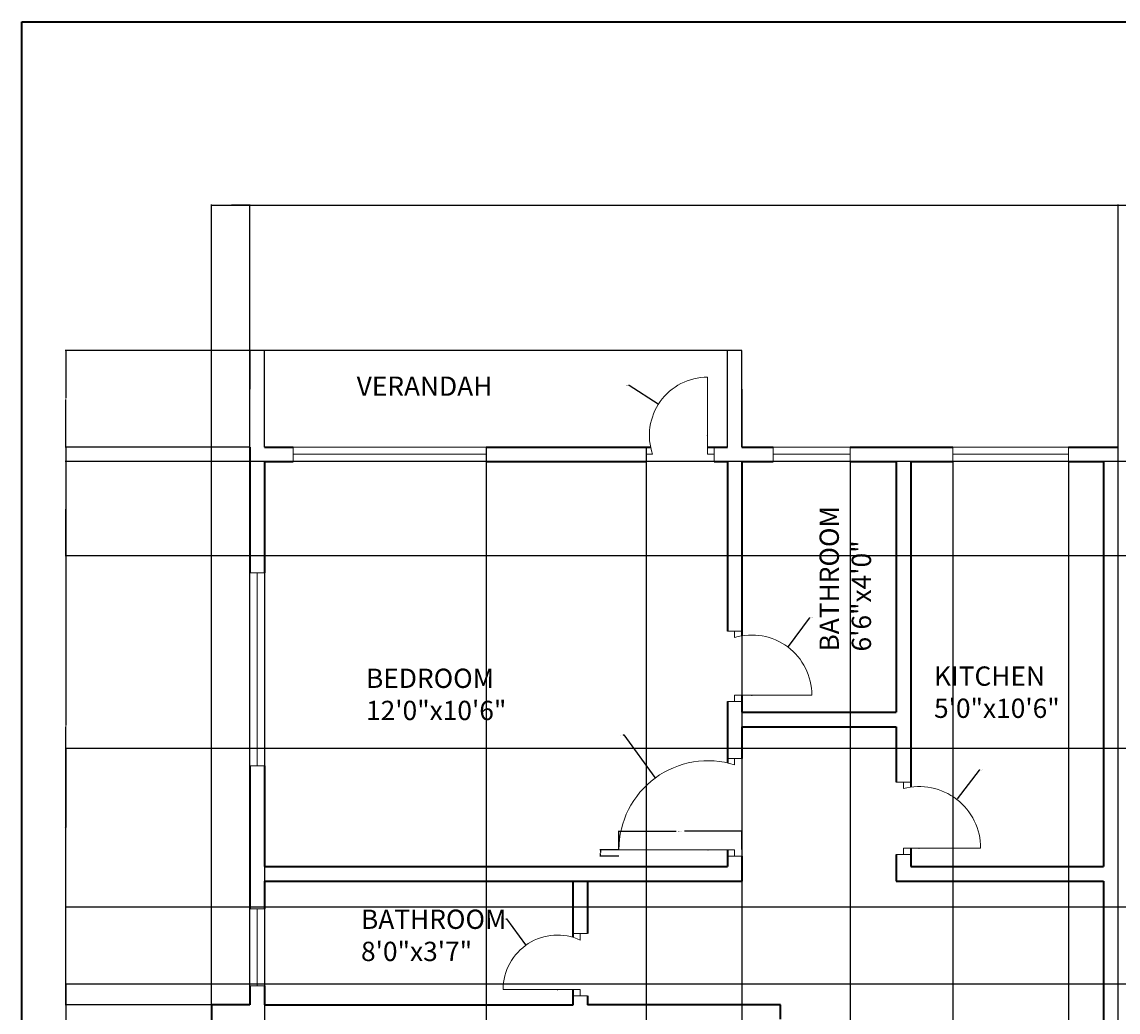
# Model space of a CAD drawing. Units: inches. Extents: x 1831 to 2867, y 1605 to 2524.
# Tile 4 of 7: x 1831 to 2172, y 2216 to 2524. Entities that reach past the tile are written whole.
import ezdxf

# ---------------------------------------------------------------- set-up
doc = ezdxf.new("R2010")
doc.units = ezdxf.units.IN
for name, color, linetype, lineweight in [('A-ANNO-DIMS', 2, 'Continuous', 18), ('A-ANNO-TTLB', 7, 'Continuous', 35), ('A-AREA-IDEN', 7, 'Continuous', 18), ('A-DOOR', 11, 'Continuous', 18), ('A-FLOR-BALC', 7, 'Continuous', 25), ('A-GLAZ', 121, 'Continuous', 18), ('A-WALL', 7, 'Continuous', 35)]:
    doc.layers.add(name, color=color, linetype=linetype, lineweight=lineweight)
doc.styles.get("Standard").update_dxf_attribs({"font": 'arial.ttf'})
doc.dimstyles.get("Standard").update_dxf_attribs({"dimtxt": 0.18, "dimasz": 0.18, "dimexe": 0.18, "dimexo": 0.0625, "dimgap": 0.09, "dimtad": 0, "dimtih": 1, "dimtoh": 1, "dimdec": 4, "dimzin": 0, "dimdsep": 46, "dimtxsty": 'Standard', "dimcen": 0.09, "dimadec": 0, "dimazin": 0, "dimtfac": 1, "dimtdec": 4, "dimtofl": 0, "dimtmove": 0, "dimatfit": 3, "dimfxl": 1, "dimtolj": 1, "dimtzin": 0, "dimarcsym": 0})

# ---------------------------------------------------------------- blocks, each defined once
blk = doc.blocks.new('WIN-60IN')
for p, q in [((4.5, 60), (0, 60)), ((0, 60), (2.25, 60)), ((0, 0), (0, 60)), ((2.25, 60), (2.25, 0)), ((4.5, 60), (4.5, 0)), ((4.5, 0), (0, 0)), ((2.25, 0), (4.5, 0))]:
    blk.add_line(p, q)
blk = doc.blocks.new('DOOR-LEAF-36IN-ALT')
for p, q in [((36, 2), (0, 2)), ((33.75, 0), (38.25, 0)), ((36, 0), (36, 2)), ((38.25, 0), (36, 0))]:
    blk.add_line(p, q)
blk = doc.blocks.new('DOOR-LEAF-24IN')
for p, q in [((2.25, 0), (2.25, 2)), ((2.25, 2), (26.25, 2)), ((0, 0), (4.5, 0)), ((4.5, 0), (2.25, 0))]:
    blk.add_line(p, q)
blk = doc.blocks.new('DOOR-LEAF-24IN-ALT')
for p, q in [((24, 2), (0, 2)), ((21.75, 0), (26.25, 0)), ((24, 0), (24, 2)), ((26.25, 0), (24, 0))]:
    blk.add_line(p, q)
blk = doc.blocks.new('DOOR-STRIKE-JAMB')
for p, q in [((0, 0), (4.5, 0)), ((2.25, 0), (2.25, 2)), ((4.5, 0), (2.25, 0))]:
    blk.add_line(p, q)
blk = doc.blocks.new('*D12')
at = {"layer": 'A-ANNO-DIMS', "color": 0, "lineweight": -2, "transparency": 16777216}
for p, q in [((2016.8, 2266.47), (2016.8, 2272.33)), ((2016.98, 2272.15), (2034.64, 2272.15)), ((2054.87, 2272.15), (2037.21, 2272.15)), ((2055.05, 2266.47), (2055.05, 2272.33))]:
    blk.add_line(p, q, dxfattribs=at)
at = {"layer": 'A-ANNO-DIMS', "color": 0, "transparency": 16777216}
for points in [[(2016.98, 2272.18), (2016.98, 2272.12), (2016.8, 2272.15)], [(2054.87, 2272.18), (2054.87, 2272.12), (2055.05, 2272.15)]]:
    blk.add_solid(points, dxfattribs=at)
at = {"layer": 'Defpoints', "color": 0, "transparency": 16777216}
for p in [(2055.05, 2272.15), (2016.8, 2266.41), (2055.05, 2266.41)]:
    blk.add_point(p, dxfattribs=at)
at = {"layer": 'A-ANNO-DIMS', "color": 0, "transparency": 16777216, "insert": (2035.93, 2272.15), "char_height": 0.18, "attachment_point": 5}
blk.add_mtext('\\A1;DOOR LEAF 38 TYP.', dxfattribs=at)
blk = doc.blocks.new('*D13')
at = {"layer": 'A-ANNO-DIMS', "color": 0, "lineweight": -2, "transparency": 16777216}
for p, q in [((2016.74, 2266.41), (2010.88, 2266.41)), ((2016.74, 2264.41), (2010.88, 2264.41)), ((2011.06, 2266.23), (2011.06, 2265.59)), ((2011.06, 2264.59), (2011.06, 2265.23))]:
    blk.add_line(p, q, dxfattribs=at)
at = {"layer": 'A-ANNO-DIMS', "color": 0, "transparency": 16777216}
for points in [[(2011.03, 2266.23), (2011.09, 2266.23), (2011.06, 2266.41)], [(2011.03, 2264.59), (2011.09, 2264.59), (2011.06, 2264.41)]]:
    blk.add_solid(points, dxfattribs=at)
at = {"layer": 'Defpoints', "color": 0, "transparency": 16777216}
for p in [(2011.06, 2266.41), (2016.8, 2266.41), (2016.8, 2264.41)]:
    blk.add_point(p, dxfattribs=at)
at = {"layer": 'A-ANNO-DIMS', "color": 0, "transparency": 16777216, "insert": (2011.06, 2265.41), "char_height": 0.18, "attachment_point": 5}
blk.add_mtext('\\A1;2 TYP.', dxfattribs=at)
blk = doc.blocks.new('*D22')
at = {"layer": 'A-ANNO-DIMS', "color": 0, "lineweight": -2, "transparency": 16777216}
for p, q in [((1890.05, 2218.24), (1890.05, 2467.15)), ((1890.23, 2466.97), (2341.22, 2466.97)), ((2792.79, 2466.97), (2341.8, 2466.97)), ((2792.97, 2421.74), (2792.97, 2467.15))]:
    blk.add_line(p, q, dxfattribs=at)
at = {"layer": 'A-ANNO-DIMS', "color": 0, "transparency": 16777216}
for points in [[(1890.23, 2467), (1890.23, 2466.94), (1890.05, 2466.97)], [(2792.79, 2467), (2792.79, 2466.94), (2792.97, 2466.97)]]:
    blk.add_solid(points, dxfattribs=at)
at = {"layer": 'Defpoints', "color": 0, "transparency": 16777216}
for p in [(2792.97, 2466.97), (2792.97, 2421.67), (1890.05, 2218.17)]:
    blk.add_point(p, dxfattribs=at)
at = {"layer": 'A-ANNO-DIMS', "color": 0, "transparency": 16777216, "insert": (2341.51, 2466.97), "char_height": 0.18, "attachment_point": 5}
blk.add_mtext('\\A1;903', dxfattribs=at)
blk = doc.blocks.new('*D31')
at = {"layer": 'A-ANNO-DIMS', "color": 0, "lineweight": -2, "transparency": 16777216}
for p, q in [((1901.99, 2421.67), (1844.57, 2421.67)), ((1844.75, 2421.49), (1844.75, 2406.86)), ((1844.75, 2391.85), (1844.75, 2406.49)), ((1901.99, 2391.67), (1844.57, 2391.67))]:
    blk.add_line(p, q, dxfattribs=at)
at = {"layer": 'A-ANNO-DIMS', "color": 0, "transparency": 16777216}
for points in [[(1844.72, 2421.49), (1844.78, 2421.49), (1844.75, 2421.67)], [(1844.72, 2391.85), (1844.78, 2391.85), (1844.75, 2391.67)]]:
    blk.add_solid(points, dxfattribs=at)
at = {"layer": 'Defpoints', "color": 0, "transparency": 16777216}
for p in [(1902.05, 2421.67), (1844.75, 2391.67), (1902.05, 2391.67)]:
    blk.add_point(p, dxfattribs=at)
at = {"layer": 'A-ANNO-DIMS', "color": 0, "transparency": 16777216, "insert": (1844.75, 2406.67), "char_height": 0.18, "attachment_point": 5}
blk.add_mtext('\\A1;30', dxfattribs=at)
blk = doc.blocks.new('*D32')
at = {"layer": 'A-ANNO-DIMS', "color": 0, "lineweight": -2, "transparency": 16777216}
for p, q in [((1901.99, 2391.67), (1844.57, 2391.67)), ((1844.75, 2391.49), (1844.75, 2305.11)), ((1844.75, 2218.35), (1844.75, 2304.74)), ((1901.99, 2218.17), (1844.57, 2218.17))]:
    blk.add_line(p, q, dxfattribs=at)
at = {"layer": 'A-ANNO-DIMS', "color": 0, "transparency": 16777216}
for points in [[(1844.72, 2391.49), (1844.78, 2391.49), (1844.75, 2391.67)], [(1844.72, 2218.35), (1844.78, 2218.35), (1844.75, 2218.17)]]:
    blk.add_solid(points, dxfattribs=at)
at = {"layer": 'Defpoints', "color": 0, "transparency": 16777216}
for p in [(1902.05, 2391.67), (1844.75, 2218.17), (1902.05, 2218.17)]:
    blk.add_point(p, dxfattribs=at)
at = {"layer": 'A-ANNO-DIMS', "color": 0, "transparency": 16777216, "insert": (1844.75, 2304.92), "char_height": 0.18, "attachment_point": 5}
blk.add_mtext('\\A1;173.5', dxfattribs=at)
blk = doc.blocks.new('*D33')
at = {"layer": 'A-ANNO-DIMS', "color": 0, "lineweight": -2, "transparency": 16777216}
for p, q in [((1889.99, 2218.17), (1844.57, 2218.17)), ((1844.75, 2217.99), (1844.75, 2093.86)), ((1844.75, 1969.35), (1844.75, 2093.49)), ((1889.99, 1969.17), (1844.57, 1969.17))]:
    blk.add_line(p, q, dxfattribs=at)
at = {"layer": 'A-ANNO-DIMS', "color": 0, "transparency": 16777216}
for points in [[(1844.72, 2217.99), (1844.78, 2217.99), (1844.75, 2218.17)], [(1844.72, 1969.35), (1844.78, 1969.35), (1844.75, 1969.17)]]:
    blk.add_solid(points, dxfattribs=at)
at = {"layer": 'Defpoints', "color": 0, "transparency": 16777216}
for p in [(1890.05, 2218.17), (1844.75, 1969.17), (1890.05, 1969.17)]:
    blk.add_point(p, dxfattribs=at)
at = {"layer": 'A-ANNO-DIMS', "color": 0, "transparency": 16777216, "insert": (1844.75, 2093.67), "char_height": 0.18, "attachment_point": 5}
blk.add_mtext('\\A1;249', dxfattribs=at)
blk = doc.blocks.new('*D36')
at = {"layer": 'A-ANNO-DIMS', "color": 0, "lineweight": -2, "transparency": 16777216}
for p, q in [((1890.05, 2218.24), (1890.05, 2467.15)), ((1890.23, 2466.97), (1895.84, 2466.97)), ((1901.87, 2466.97), (1896.26, 2466.97)), ((1902.05, 2218.24), (1902.05, 2467.15))]:
    blk.add_line(p, q, dxfattribs=at)
at = {"layer": 'A-ANNO-DIMS', "color": 0, "transparency": 16777216}
for points in [[(1890.23, 2467), (1890.23, 2466.94), (1890.05, 2466.97)], [(1901.87, 2467), (1901.87, 2466.94), (1902.05, 2466.97)]]:
    blk.add_solid(points, dxfattribs=at)
at = {"layer": 'Defpoints', "color": 0, "transparency": 16777216}
for p in [(1902.05, 2466.97), (1890.05, 2218.17), (1902.05, 2218.17)]:
    blk.add_point(p, dxfattribs=at)
at = {"layer": 'A-ANNO-DIMS', "color": 0, "transparency": 16777216, "insert": (1896.05, 2466.97), "char_height": 0.18, "attachment_point": 5}
blk.add_mtext('\\A1;12', dxfattribs=at)
blk = doc.blocks.new('*D37')
at = {"layer": 'A-ANNO-DIMS', "color": 0, "lineweight": -2, "transparency": 16777216}
for p, q in [((1906.55, 2387.11), (1906.55, 1715.69)), ((1975.47, 2387.11), (1975.47, 1715.69)), ((1906.73, 1715.87), (1940.62, 1715.87)), ((1975.29, 1715.87), (1941.4, 1715.87))]:
    blk.add_line(p, q, dxfattribs=at)
at = {"layer": 'A-ANNO-DIMS', "color": 0, "transparency": 16777216}
for points in [[(1906.73, 1715.9), (1906.73, 1715.84), (1906.55, 1715.87)], [(1975.29, 1715.9), (1975.29, 1715.84), (1975.47, 1715.87)]]:
    blk.add_solid(points, dxfattribs=at)
at = {"layer": 'Defpoints', "color": 0, "transparency": 16777216}
for p in [(1906.55, 2387.17), (1975.47, 2387.17), (1975.47, 1715.87)]:
    blk.add_point(p, dxfattribs=at)
at = {"layer": 'A-ANNO-DIMS', "color": 0, "transparency": 16777216, "insert": (1941.01, 1715.87), "char_height": 0.18, "attachment_point": 5}
blk.add_mtext('\\A1;68.92', dxfattribs=at)
blk = doc.blocks.new('*D38')
at = {"layer": 'A-ANNO-DIMS', "color": 0, "lineweight": -2, "transparency": 16777216}
for p, q in [((1975.47, 2391.61), (1975.47, 1715.69)), ((2025.28, 2391.61), (2025.28, 1715.69)), ((1975.65, 1715.87), (1999.99, 1715.87)), ((2025.1, 1715.87), (2000.75, 1715.87))]:
    blk.add_line(p, q, dxfattribs=at)
at = {"layer": 'A-ANNO-DIMS', "color": 0, "transparency": 16777216}
for points in [[(1975.65, 1715.9), (1975.65, 1715.84), (1975.47, 1715.87)], [(2025.1, 1715.9), (2025.1, 1715.84), (2025.28, 1715.87)]]:
    blk.add_solid(points, dxfattribs=at)
at = {"layer": 'Defpoints', "color": 0, "transparency": 16777216}
for p in [(1975.47, 2391.67), (2025.28, 2391.67), (2025.28, 1715.87)]:
    blk.add_point(p, dxfattribs=at)
at = {"layer": 'A-ANNO-DIMS', "color": 0, "transparency": 16777216, "insert": (2000.37, 1715.87), "char_height": 0.18, "attachment_point": 5}
blk.add_mtext('\\A1;49.81', dxfattribs=at)
blk = doc.blocks.new('*D39')
at = {"layer": 'A-ANNO-DIMS', "color": 0, "lineweight": -2, "transparency": 16777216}
for p, q in [((2055.05, 2387.11), (2055.05, 1715.69)), ((2088.73, 2387.11), (2088.73, 1715.69)), ((2055.23, 1715.87), (2071.5, 1715.87)), ((2088.55, 1715.87), (2072.28, 1715.87))]:
    blk.add_line(p, q, dxfattribs=at)
at = {"layer": 'A-ANNO-DIMS', "color": 0, "transparency": 16777216}
for points in [[(2055.23, 1715.9), (2055.23, 1715.84), (2055.05, 1715.87)], [(2088.55, 1715.9), (2088.55, 1715.84), (2088.73, 1715.87)]]:
    blk.add_solid(points, dxfattribs=at)
at = {"layer": 'Defpoints', "color": 0, "transparency": 16777216}
for p in [(2055.05, 2387.17), (2088.73, 2387.17), (2088.73, 1715.87)]:
    blk.add_point(p, dxfattribs=at)
at = {"layer": 'A-ANNO-DIMS', "color": 0, "transparency": 16777216, "insert": (2071.89, 1715.87), "char_height": 0.18, "attachment_point": 5}
blk.add_mtext('\\A1;33.68', dxfattribs=at)
blk = doc.blocks.new('*D40')
at = {"layer": 'A-ANNO-DIMS', "color": 0, "lineweight": -2, "transparency": 16777216}
for p, q in [((2088.73, 2387.11), (2088.73, 1715.69)), ((2120.64, 2387.11), (2120.64, 1715.69)), ((2088.91, 1715.87), (2104.31, 1715.87)), ((2120.46, 1715.87), (2105.06, 1715.87))]:
    blk.add_line(p, q, dxfattribs=at)
at = {"layer": 'A-ANNO-DIMS', "color": 0, "transparency": 16777216}
for points in [[(2088.91, 1715.9), (2088.91, 1715.84), (2088.73, 1715.87)], [(2120.46, 1715.9), (2120.46, 1715.84), (2120.64, 1715.87)]]:
    blk.add_solid(points, dxfattribs=at)
at = {"layer": 'Defpoints', "color": 0, "transparency": 16777216}
for p in [(2088.73, 2387.17), (2120.64, 2387.17), (2120.64, 1715.87)]:
    blk.add_point(p, dxfattribs=at)
at = {"layer": 'A-ANNO-DIMS', "color": 0, "transparency": 16777216, "insert": (2104.69, 1715.87), "char_height": 0.18, "attachment_point": 5}
blk.add_mtext('\\A1;31.91', dxfattribs=at)
blk = doc.blocks.new('*D41')
at = {"layer": 'A-ANNO-DIMS', "color": 0, "lineweight": -2, "transparency": 16777216}
for p, q in [((2156.64, 2387.11), (2156.64, 1715.69)), ((2210.17, 2387.11), (2210.17, 1715.69)), ((2156.82, 1715.87), (2183.01, 1715.87)), ((2209.99, 1715.87), (2183.8, 1715.87))]:
    blk.add_line(p, q, dxfattribs=at)
at = {"layer": 'A-ANNO-DIMS', "color": 0, "transparency": 16777216}
for points in [[(2156.82, 1715.9), (2156.82, 1715.84), (2156.64, 1715.87)], [(2209.99, 1715.9), (2209.99, 1715.84), (2210.17, 1715.87)]]:
    blk.add_solid(points, dxfattribs=at)
at = {"layer": 'Defpoints', "color": 0, "transparency": 16777216}
for p in [(2156.64, 2387.17), (2210.17, 2387.17), (2210.17, 1715.87)]:
    blk.add_point(p, dxfattribs=at)
at = {"layer": 'A-ANNO-DIMS', "color": 0, "transparency": 16777216, "insert": (2183.4, 1715.87), "char_height": 0.18, "attachment_point": 5}
blk.add_mtext('\\A1;53.52', dxfattribs=at)
blk = doc.blocks.new('*D49')
at = {"layer": 'A-ANNO-DIMS', "color": 0, "lineweight": -2, "transparency": 16777216}
for p, q in [((2786.99, 2387.17), (1844.57, 2387.17)), ((1844.75, 2386.99), (1844.75, 2372.7)), ((1844.75, 2358.05), (1844.75, 2372.34)), ((2786.99, 2357.87), (1844.57, 2357.87))]:
    blk.add_line(p, q, dxfattribs=at)
at = {"layer": 'A-ANNO-DIMS', "color": 0, "transparency": 16777216}
for points in [[(1844.72, 2386.99), (1844.78, 2386.99), (1844.75, 2387.17)], [(1844.72, 2358.05), (1844.78, 2358.05), (1844.75, 2357.87)]]:
    blk.add_solid(points, dxfattribs=at)
at = {"layer": 'Defpoints', "color": 0, "transparency": 16777216}
for p in [(2787.05, 2387.17), (1844.75, 2357.87), (2787.05, 2357.87)]:
    blk.add_point(p, dxfattribs=at)
at = {"layer": 'A-ANNO-DIMS', "color": 0, "transparency": 16777216, "insert": (1844.75, 2372.52), "char_height": 0.18, "attachment_point": 5}
blk.add_mtext('\\A1;29.31', dxfattribs=at)
blk = doc.blocks.new('*D50')
at = {"layer": 'A-ANNO-DIMS', "color": 0, "lineweight": -2, "transparency": 16777216}
for p, q in [((2786.99, 2297.87), (1844.57, 2297.87)), ((1844.75, 2297.69), (1844.75, 2273.42)), ((1844.75, 2248.78), (1844.75, 2273.05)), ((2786.99, 2248.6), (1844.57, 2248.6))]:
    blk.add_line(p, q, dxfattribs=at)
at = {"layer": 'A-ANNO-DIMS', "color": 0, "transparency": 16777216}
for points in [[(1844.72, 2297.69), (1844.78, 2297.69), (1844.75, 2297.87)], [(1844.72, 2248.78), (1844.78, 2248.78), (1844.75, 2248.6)]]:
    blk.add_solid(points, dxfattribs=at)
at = {"layer": 'Defpoints', "color": 0, "transparency": 16777216}
for p in [(2787.05, 2297.87), (1844.75, 2248.6), (2787.05, 2248.6)]:
    blk.add_point(p, dxfattribs=at)
at = {"layer": 'A-ANNO-DIMS', "color": 0, "transparency": 16777216, "insert": (1844.75, 2273.23), "char_height": 0.18, "attachment_point": 5}
blk.add_mtext('\\A1;49.26', dxfattribs=at)
blk = doc.blocks.new('*D51')
at = {"layer": 'A-ANNO-DIMS', "color": 0, "lineweight": -2, "transparency": 16777216}
for p, q in [((2786.99, 2224.6), (1844.57, 2224.6)), ((1844.75, 2224.42), (1844.75, 2206.21)), ((1844.75, 2187.63), (1844.75, 2205.85)), ((2786.99, 2187.45), (1844.57, 2187.45))]:
    blk.add_line(p, q, dxfattribs=at)
at = {"layer": 'A-ANNO-DIMS', "color": 0, "transparency": 16777216}
for points in [[(1844.72, 2224.42), (1844.78, 2224.42), (1844.75, 2224.6)], [(1844.72, 2187.63), (1844.78, 2187.63), (1844.75, 2187.45)]]:
    blk.add_solid(points, dxfattribs=at)
at = {"layer": 'Defpoints', "color": 0, "transparency": 16777216}
for p in [(2787.05, 2224.6), (1844.75, 2187.45), (2787.05, 2187.45)]:
    blk.add_point(p, dxfattribs=at)
at = {"layer": 'A-ANNO-DIMS', "color": 0, "transparency": 16777216, "insert": (1844.75, 2206.03), "char_height": 0.18, "attachment_point": 5}
blk.add_mtext('\\A1;37.15', dxfattribs=at)
blk = doc.blocks.new('*D63')
at = {"layer": 'A-ANNO-DIMS', "color": 0, "lineweight": -2, "transparency": 16777216}
for p, q in [((2172.05, 1795.74), (2172.05, 2467.15)), ((2172.23, 2466.97), (2183.83, 2466.97)), ((2195.87, 2466.97), (2184.27, 2466.97)), ((2196.05, 1795.74), (2196.05, 2467.15))]:
    blk.add_line(p, q, dxfattribs=at)
at = {"layer": 'A-ANNO-DIMS', "color": 0, "transparency": 16777216}
for points in [[(2172.23, 2467), (2172.23, 2466.94), (2172.05, 2466.97)], [(2195.87, 2467), (2195.87, 2466.94), (2196.05, 2466.97)]]:
    blk.add_solid(points, dxfattribs=at)
at = {"layer": 'Defpoints', "color": 0, "transparency": 16777216}
for p in [(2196.05, 2466.97), (2172.05, 1795.67), (2196.05, 1795.67)]:
    blk.add_point(p, dxfattribs=at)
at = {"layer": 'A-ANNO-DIMS', "color": 0, "transparency": 16777216, "insert": (2184.05, 2466.97), "char_height": 0.18, "attachment_point": 5}
blk.add_mtext('\\A1;24', dxfattribs=at)
blk = doc.blocks.new('*D75')
at = {"layer": 'A-ANNO-DIMS', "color": 0, "lineweight": -2, "transparency": 16777216}
for p, q in [((2018.1, 2302.13), (2018.28, 2302.13)), ((2018.28, 2302.13), (2028, 2288.88)), ((2044.41, 2266.41), (2044.59, 2266.41)), ((2044.5, 2266.32), (2044.5, 2266.5))]:
    blk.add_line(p, q, dxfattribs=at)
at = {"layer": 'A-ANNO-DIMS', "color": 0, "transparency": 16777216}
blk.add_solid([(2028.03, 2288.9), (2027.98, 2288.86), (2028.11, 2288.74)], dxfattribs=at)
at = {"layer": 'Defpoints', "color": 0, "transparency": 16777216}
for p in [(2028.11, 2288.74), (2044.5, 2266.41)]:
    blk.add_point(p, dxfattribs=at)
at = {"layer": 'A-ANNO-DIMS', "color": 0, "transparency": 16777216, "insert": (2017.55, 2302.13), "char_height": 0.18, "attachment_point": 5}
blk.add_mtext('\\A1;R27.694', dxfattribs=at)
blk = doc.blocks.new('*D88')
at = {"layer": 'A-ANNO-DIMS', "color": 0, "lineweight": -2, "transparency": 16777216}
for p, q in [((2128.89, 2291.19), (2121.96, 2282.24)), ((2129.07, 2291.19), (2128.89, 2291.19)), ((2110.04, 2266.93), (2110.22, 2266.93)), ((2110.13, 2266.84), (2110.13, 2267.02))]:
    blk.add_line(p, q, dxfattribs=at)
at = {"layer": 'A-ANNO-DIMS', "color": 0, "transparency": 16777216}
blk.add_solid([(2121.94, 2282.25), (2121.99, 2282.22), (2121.85, 2282.09)], dxfattribs=at)
at = {"layer": 'Defpoints', "color": 0, "transparency": 16777216}
for p in [(2121.85, 2282.09), (2110.13, 2266.93)]:
    blk.add_point(p, dxfattribs=at)
at = {"layer": 'A-ANNO-DIMS', "color": 0, "transparency": 16777216, "insert": (2129.62, 2291.19), "char_height": 0.18, "attachment_point": 5}
blk.add_mtext('\\A1;R19.168', dxfattribs=at)
blk = doc.blocks.new('*D93')
at = {"layer": 'A-ANNO-DIMS', "color": 0, "lineweight": -2, "transparency": 16777216}
for p, q in [((2075.99, 2338.48), (2069.4, 2329.65)), ((2076.17, 2338.48), (2075.99, 2338.48)), ((2058.04, 2314.53), (2058.22, 2314.53)), ((2058.13, 2314.44), (2058.13, 2314.62))]:
    blk.add_line(p, q, dxfattribs=at)
at = {"layer": 'A-ANNO-DIMS', "color": 0, "transparency": 16777216}
blk.add_solid([(2069.37, 2329.66), (2069.42, 2329.63), (2069.29, 2329.5)], dxfattribs=at)
at = {"layer": 'Defpoints', "color": 0, "transparency": 16777216}
for p in [(2069.29, 2329.5), (2058.13, 2314.53)]:
    blk.add_point(p, dxfattribs=at)
at = {"layer": 'A-ANNO-DIMS', "color": 0, "transparency": 16777216, "insert": (2076.72, 2338.48), "char_height": 0.18, "attachment_point": 5}
blk.add_mtext('\\A1;R18.675', dxfattribs=at)
blk = doc.blocks.new('*D95')
at = {"layer": 'A-ANNO-DIMS', "color": 0, "lineweight": -2, "transparency": 16777216}
for p, q in [((1981.68, 2244.91), (1981.86, 2244.91)), ((1981.86, 2244.91), (1987.71, 2236.82)), ((1997.63, 2222.96), (1997.81, 2222.96)), ((1997.72, 2222.87), (1997.72, 2223.05))]:
    blk.add_line(p, q, dxfattribs=at)
at = {"layer": 'A-ANNO-DIMS', "color": 0, "transparency": 16777216}
blk.add_solid([(1987.73, 2236.84), (1987.68, 2236.81), (1987.81, 2236.68)], dxfattribs=at)
at = {"layer": 'Defpoints', "color": 0, "transparency": 16777216}
for p in [(1987.81, 2236.68), (1997.72, 2222.96)]:
    blk.add_point(p, dxfattribs=at)
at = {"layer": 'A-ANNO-DIMS', "color": 0, "transparency": 16777216, "insert": (1981.13, 2244.91), "char_height": 0.18, "attachment_point": 5}
blk.add_mtext('\\A1;R16.924', dxfattribs=at)
blk = doc.blocks.new('*D105')
at = {"layer": 'A-ANNO-DIMS', "color": 0, "lineweight": -2, "transparency": 16777216}
for p, q in [((2019.79, 2410.9), (2019.97, 2410.9)), ((2019.97, 2410.9), (2028.97, 2405.16)), ((2044.29, 2395.33), (2044.47, 2395.33)), ((2044.38, 2395.24), (2044.38, 2395.42))]:
    blk.add_line(p, q, dxfattribs=at)
at = {"layer": 'A-ANNO-DIMS', "color": 0, "transparency": 16777216}
blk.add_solid([(2028.99, 2405.18), (2028.95, 2405.13), (2029.12, 2405.06)], dxfattribs=at)
at = {"layer": 'Defpoints', "color": 0, "transparency": 16777216}
for p in [(2029.12, 2405.06), (2044.38, 2395.33)]:
    blk.add_point(p, dxfattribs=at)
at = {"layer": 'A-ANNO-DIMS', "color": 0, "transparency": 16777216, "insert": (2019.24, 2410.9), "char_height": 0.18, "attachment_point": 5}
blk.add_mtext('\\A1;R18.093', dxfattribs=at)

msp = doc.modelspace()

# ---------------------------------------------------------------- linework, layer by layer
at = {"layer": 'A-ANNO-TTLB'}
msp.add_lwpolyline([(1831.1248, 2523.9204), (2867.0416, 2523.9204), (2867.0416, 1605.0781), (1831.1248, 1605.0781)], close=True, dxfattribs=at)
at = {"layer": 'A-DOOR'}
for centre, radius, start, end in [((2044.3763, 2395.3312), 18.0926, 90, 199.057127), ((2058.1262, 2314.5317), 18.6748, 360, 106.567926), ((2044.495, 2266.4091), 27.694, 72.547245, 180), ((2110.1331, 2266.9265), 19.1679, 0, 104.601409), ((1997.7246, 2222.9608), 16.9236, 65.282987, 180)]:
    msp.add_arc(centre, radius, start, end, dxfattribs=at)
at = {"layer": 'A-FLOR-BALC'}
for p, q in [((2055.051, 2421.6738), (1902.051, 2421.6738)), ((1902.051, 2421.6738), (1902.051, 2409.6738)), ((1906.551, 2391.6738), (1906.551, 2421.6738)), ((2050.551, 2391.6738), (2050.551, 2421.6738)), ((2055.051, 2415.6738), (2055.051, 2421.6738)), ((2055.051, 2391.6738), (2055.051, 2415.6738)), ((1902.051, 2391.6738), (1902.051, 2409.6738)), ((2055.051, 2409.6738), (2055.051, 2391.6738))]:
    msp.add_line(p, q, dxfattribs=at)
at = {"layer": 'A-GLAZ'}
for p, q in [((2064.7306, 2387.1738), (2064.7306, 2391.6738)), ((2064.7306, 2391.6738), (2064.7306, 2389.4238)), ((2088.7306, 2391.6738), (2064.7306, 2391.6738)), ((2088.7306, 2389.4238), (2088.7306, 2391.6738)), ((2088.7306, 2391.6738), (2088.7306, 2387.1738)), ((2120.6429, 2387.1738), (2120.6429, 2391.6738)), ((2120.6429, 2391.6738), (2120.6429, 2389.4238)), ((2156.6429, 2391.6738), (2120.6429, 2391.6738)), ((2156.6429, 2389.4238), (2156.6429, 2391.6738)), ((2156.6429, 2391.6738), (2156.6429, 2387.1738)), ((2064.7306, 2389.4238), (2088.7306, 2389.4238)), ((2064.7306, 2387.1738), (2088.7306, 2387.1738)), ((2120.6429, 2389.4238), (2156.6429, 2389.4238)), ((2120.6429, 2387.1738), (2156.6429, 2387.1738)), ((1904.301, 2352.544), (1902.051, 2352.544)), ((1902.051, 2352.544), (1906.551, 2352.544)), ((1902.051, 2352.544), (1902.051, 2292.544)), ((1904.301, 2328.544), (1904.301, 2352.544)), ((1906.551, 2352.544), (1906.551, 2292.544)), ((1904.301, 2292.544), (1904.301, 2328.544)), ((1902.051, 2292.544), (1906.551, 2292.544)), ((1906.551, 2292.544), (1904.301, 2292.544)), ((1904.301, 2248.0694), (1902.051, 2248.0694)), ((1902.051, 2248.0694), (1906.551, 2248.0694)), ((1902.051, 2248.0694), (1902.051, 2224.0694)), ((1904.301, 2224.0694), (1904.301, 2248.0694)), ((1906.551, 2248.0694), (1906.551, 2224.0694)), ((1902.051, 2224.0694), (1906.551, 2224.0694)), ((1906.551, 2224.0694), (1902.051, 2224.0694))]:
    msp.add_line(p, q, dxfattribs=at)
at = {"layer": 'A-WALL'}
for p, q in [((1902.051, 2391.6738), (1902.051, 2352.544)), ((1906.551, 2391.6738), (1915.4676, 2391.6738)), ((1975.4676, 2391.6738), (2026.6572, 2391.6738)), ((2044.3763, 2391.6738), (2050.551, 2391.6738)), ((2055.051, 2391.6738), (2064.7306, 2391.6738)), ((2088.7306, 2391.6738), (2120.6429, 2391.6738)), ((2156.6429, 2391.6738), (2172.051, 2391.6738)), ((1906.551, 2387.1738), (1915.4676, 2387.1738)), ((1906.551, 2387.1738), (1906.551, 2352.544)), ((1975.4676, 2387.1738), (2025.2753, 2387.1738)), ((2046.3763, 2387.1738), (2050.551, 2387.1738)), ((2050.551, 2387.1738), (2050.551, 2334.4312)), ((2055.051, 2387.1738), (2055.051, 2332.9516)), ((2055.051, 2387.1738), (2064.7306, 2387.1738)), ((2088.7306, 2387.1738), (2103.051, 2387.1738)), ((2103.051, 2387.1738), (2103.051, 2309.1738)), ((2107.551, 2387.1738), (2107.551, 2285.9196)), ((2107.551, 2387.1738), (2120.6429, 2387.1738)), ((2156.6429, 2387.1738), (2167.551, 2387.1738)), ((2167.551, 2387.1738), (2167.551, 2261.1738)), ((2050.551, 2312.5317), (2050.551, 2293.4329)), ((2055.051, 2314.5317), (2055.051, 2309.1738)), ((2055.051, 2309.1738), (2103.051, 2309.1738)), ((2055.051, 2304.6738), (2103.051, 2304.6738)), ((2055.051, 2304.6738), (2055.051, 2294.8283)), ((2103.051, 2304.6738), (2103.051, 2287.4753)), ((1902.051, 2292.544), (1902.051, 2248.0694)), ((1906.551, 2292.544), (1906.551, 2261.1738)), ((2050.551, 2266.4091), (2050.551, 2261.1738)), ((2055.051, 2264.4091), (2055.051, 2256.6738)), ((2103.051, 2264.9265), (2103.051, 2256.6738)), ((2107.551, 2266.9265), (2107.551, 2261.1738)), ((1906.551, 2261.1738), (2050.551, 2261.1738)), ((2107.551, 2261.1738), (2167.551, 2261.1738)), ((1906.551, 2256.6738), (2055.051, 2256.6738)), ((1906.551, 2256.6738), (1906.551, 2248.0694)), ((1906.551, 2256.6738), (1906.551, 2248.0694)), ((2002.551, 2256.6738), (2007.051, 2256.6738)), ((2002.551, 2239.1816), (2002.551, 2256.6738)), ((2007.051, 2256.6738), (2007.051, 2240.3339)), ((2103.051, 2256.6738), (2167.551, 2256.6738)), ((2167.551, 2256.6738), (2167.551, 2127.6074)), ((1902.051, 2224.0694), (1902.051, 2218.1738)), ((1906.551, 2224.0694), (1906.551, 2218.1738)), ((1906.551, 2224.0694), (1906.551, 2218.1738)), ((2002.551, 2218.1738), (2002.551, 2222.9608)), ((2007.051, 2220.9608), (2007.051, 2218.1738)), ((1902.051, 2218.1738), (1890.051, 2218.1738)), ((1890.051, 2218.1738), (1890.051, 2177.8352)), ((1906.551, 2218.1738), (2002.551, 2218.1738)), ((2067.051, 2218.1738), (2007.051, 2218.1738)), ((2067.051, 2213.6738), (2067.051, 2218.1738))]:
    msp.add_line(p, q, dxfattribs=at)

# ---------------------------------------------------------------- block references
at = {"layer": 'A-DOOR', "extrusion": (0, 0, -1), "zscale": -1}
for name, p, rotation in [('DOOR-LEAF-24IN-ALT', (-2046.3763, 2413.4238), 269.9999999999994), ('DOOR-STRIKE-JAMB', (-2050.551, 2334.4312), 180), ('DOOR-STRIKE-JAMB', (-2050.551, 2294.8283), 180), ('DOOR-STRIKE-JAMB', (-2103.051, 2287.4753), 180), ('DOOR-STRIKE-JAMB', (-2002.551, 2240.3339), 180)]:
    msp.add_blockref(name, p, dxfattribs=dict(at, rotation=rotation))
at = {"layer": 'A-DOOR', "rotation": 270.0000000000085}
msp.add_blockref('DOOR-STRIKE-JAMB', (2025.2753, 2391.6738), dxfattribs=at)
at = {"layer": 'A-DOOR'}
for name, p in [('DOOR-LEAF-24IN', (2050.551, 2312.5317)), ('DOOR-LEAF-36IN-ALT', (2016.801, 2264.4091)), ('DOOR-LEAF-24IN', (2103.051, 2264.9265)), ('DOOR-LEAF-24IN-ALT', (1980.801, 2220.9608))]:
    msp.add_blockref(name, p, dxfattribs=at)
at = {"layer": 'A-GLAZ', "rotation": 89.9999999999992}
msp.add_blockref('WIN-60IN', (1975.4676, 2387.1738), dxfattribs=at)

# ---------------------------------------------------------------- texts
at = {"layer": 'A-AREA-IDEN', "char_height": 6, "attachment_point": 1}
for s, width, insert in [('VERANDAH', 121.894867, (1935.2447, 2413.62)), ('BEDROOM\\P12\'0"x10\'6"', 112.305244, (1938.1516, 2322.7479)), ('KITCHEN\\P5\'0"x10\'6"', 95.123911, (2114.8009, 2323.4351)), ('BATHROOM\\P8\'0"x3\'7"', 112.574307, (1936.5876, 2247.7963))]:
    msp.add_mtext_dynamic_manual_height_columns(s, width=width, gutter_width=12.5, heights=[0], dxfattribs=dict(at, insert=insert))
at = {"layer": 'A-AREA-IDEN', "insert": (2079.2117, 2328.0888), "char_height": 6, "attachment_point": 1, "rotation": 90}
msp.add_mtext_dynamic_manual_height_columns('BATHROOM\\P6\'6"x4\'0"', width=61.408145, gutter_width=12.5, heights=[0], dxfattribs=at)

# ---------------------------------------------------------------- dimensions: what is measured, and where the dimension line sits
at = {"layer": 'A-ANNO-DIMS'}
for base, p1, p2, override, picture, middle in [((2792.9663, 2466.9738), (1890.051, 2218.1738), (2792.9663, 2421.6738), {"dimdec": 0, "dimlfac": 1, "dimrnd": 0, "dimzin": 0, "dimdsep": 46, "dimlunit": 2}, '*D22', (2341.5086, 2466.9738)), ((1902.051, 2466.9738), (1890.051, 2218.1738), (1902.051, 2218.1738), {"dimdec": 0, "dimlfac": 1, "dimrnd": 0, "dimzin": 0, "dimdsep": 46, "dimlunit": 2}, '*D36', (1896.051, 2466.9738)), ((2196.051, 2466.9738), (2172.051, 1795.6738), (2196.051, 1795.6738), {"dimdec": 0, "dimlfac": 1, "dimrnd": 0, "dimzin": 0, "dimdsep": 46, "dimlunit": 2}, '*D63', (2184.051, 2466.9738)), ((2025.2753, 1715.8738), (1975.4676, 2391.6738), (2025.2753, 2391.6738), {"dimdec": 2, "dimlfac": 1, "dimrnd": 0, "dimzin": 0, "dimdsep": 46, "dimlunit": 2}, '*D38', (2000.3714, 1715.8738)), ((1975.4676, 1715.8738), (1906.551, 2387.1738), (1975.4676, 2387.1738), {"dimdec": 2, "dimlfac": 1, "dimrnd": 0, "dimzin": 0, "dimdsep": 46, "dimlunit": 2}, '*D37', (1941.0093, 1715.8738)), ((2088.7306, 1715.8738), (2055.051, 2387.1738), (2088.7306, 2387.1738), {"dimdec": 2, "dimlfac": 1, "dimrnd": 0, "dimzin": 0, "dimdsep": 46, "dimlunit": 2}, '*D39', (2071.8908, 1715.8738)), ((2120.6429, 1715.8738), (2088.7306, 2387.1738), (2120.6429, 2387.1738), {"dimdec": 2, "dimlfac": 1, "dimrnd": 0, "dimzin": 0, "dimdsep": 46, "dimlunit": 2}, '*D40', (2104.6867, 1715.8738)), ((2210.1653, 1715.8738), (2156.6429, 2387.1738), (2210.1653, 2387.1738), {"dimdec": 2, "dimlfac": 1, "dimrnd": 0, "dimzin": 0, "dimdsep": 46, "dimlunit": 2}, '*D41', (2183.4041, 1715.8738))]:
    dim = msp.add_linear_dim(base=base, p1=p1, p2=p2, dimstyle='Standard', override=override, dxfattribs=at)
    dim.commit()
    dim.dimension.update_dxf_attribs({"geometry": picture, "text_midpoint": middle})
for base, p1, p2, override, picture, middle in [((1844.751, 2391.6738), (1902.051, 2421.6738), (1902.051, 2391.6738), {"dimdec": 0, "dimlfac": 1, "dimrnd": 0, "dimzin": 0, "dimdsep": 46, "dimlunit": 2}, '*D31', (1844.751, 2406.6738)), ((1844.751, 2218.1738), (1902.051, 2391.6738), (1902.051, 2218.1738), {"dimdec": 1, "dimlfac": 1, "dimrnd": 0, "dimzin": 0, "dimdsep": 46, "dimlunit": 2}, '*D32', (1844.751, 2304.9238)), ((1844.751, 2357.8655), (2787.051, 2387.1738), (2787.051, 2357.8655), {"dimdec": 2, "dimlfac": 1, "dimrnd": 0, "dimzin": 0, "dimdsep": 46, "dimlunit": 2}, '*D49', (1844.751, 2372.5196)), ((1844.751, 2248.6027), (2787.051, 2297.8655), (2787.051, 2248.6027), {"dimdec": 2, "dimlfac": 1, "dimrnd": 0, "dimzin": 0, "dimdsep": 46, "dimlunit": 2}, '*D50', (1844.751, 2273.2341)), ((1844.751, 2187.452), (2787.051, 2224.6027), (2787.051, 2187.452), {"dimdec": 2, "dimlfac": 1, "dimrnd": 0, "dimzin": 0, "dimdsep": 46, "dimlunit": 2}, '*D51', (1844.751, 2206.0273)), ((1844.751, 1969.1738), (1890.051, 2218.1738), (1890.051, 1969.1738), {"dimdec": 0, "dimlfac": 1, "dimrnd": 0, "dimzin": 0, "dimdsep": 46, "dimlunit": 2}, '*D33', (1844.751, 2093.6738))]:
    dim = msp.add_linear_dim(base=base, p1=p1, p2=p2, angle=90, dimstyle='Standard', override=override, dxfattribs=at)
    dim.commit()
    dim.dimension.update_dxf_attribs({"geometry": picture, "text_midpoint": middle})
for center, mpoint, picture, middle in [((2044.3763, 2395.3312), (2029.122, 2405.06), '*D105', (2019.2397, 2410.8972)), ((2058.1262, 2314.5317), (2069.2908, 2329.5017), '*D93', (2076.72, 2338.4837)), ((2044.495, 2266.4091), (2028.11, 2288.736), '*D75', (2017.5496, 2302.1321)), ((2110.1331, 2266.9265), (2121.8547, 2282.0926), '*D88', (2129.6176, 2291.1923)), ((1997.7246, 2222.9608), (1987.8115, 2236.6772), '*D95', (1981.1342, 2244.907))]:
    dim = msp.add_radius_dim(center=center, mpoint=mpoint, dimstyle='Standard', override={"dimdec": 3, "dimlfac": 1, "dimrnd": 0, "dimzin": 0, "dimdsep": 46, "dimlunit": 2}, dxfattribs=at)
    dim.commit()
    dim.dimension.update_dxf_attribs({"geometry": picture, "text_midpoint": middle, "dimtype": 164})
dim = msp.add_linear_dim(base=(2055.051, 2272.1466), p1=(2016.801, 2266.4091), p2=(2055.051, 2266.4091), text='DOOR LEAF <> TYP.', dimstyle='Standard', override={"dimdec": 0, "dimlfac": 1, "dimrnd": 0, "dimzin": 0, "dimdsep": 46, "dimlunit": 2}, dxfattribs=at)
dim.commit()
dim.dimension.update_dxf_attribs({"geometry": '*D12', "text_midpoint": (2035.926, 2272.1466)})
dim = msp.add_linear_dim(base=(2011.0635, 2266.4091), p1=(2016.801, 2264.4091), p2=(2016.801, 2266.4091), angle=90, text='<> TYP.', dimstyle='Standard', override={"dimdec": 0, "dimlfac": 1, "dimrnd": 0, "dimzin": 0, "dimdsep": 46, "dimlunit": 2}, dxfattribs=at)
dim.commit()
dim.dimension.update_dxf_attribs({"geometry": '*D13', "text_midpoint": (2011.0635, 2265.4091)})

doc.saveas('drawing.dxf')
